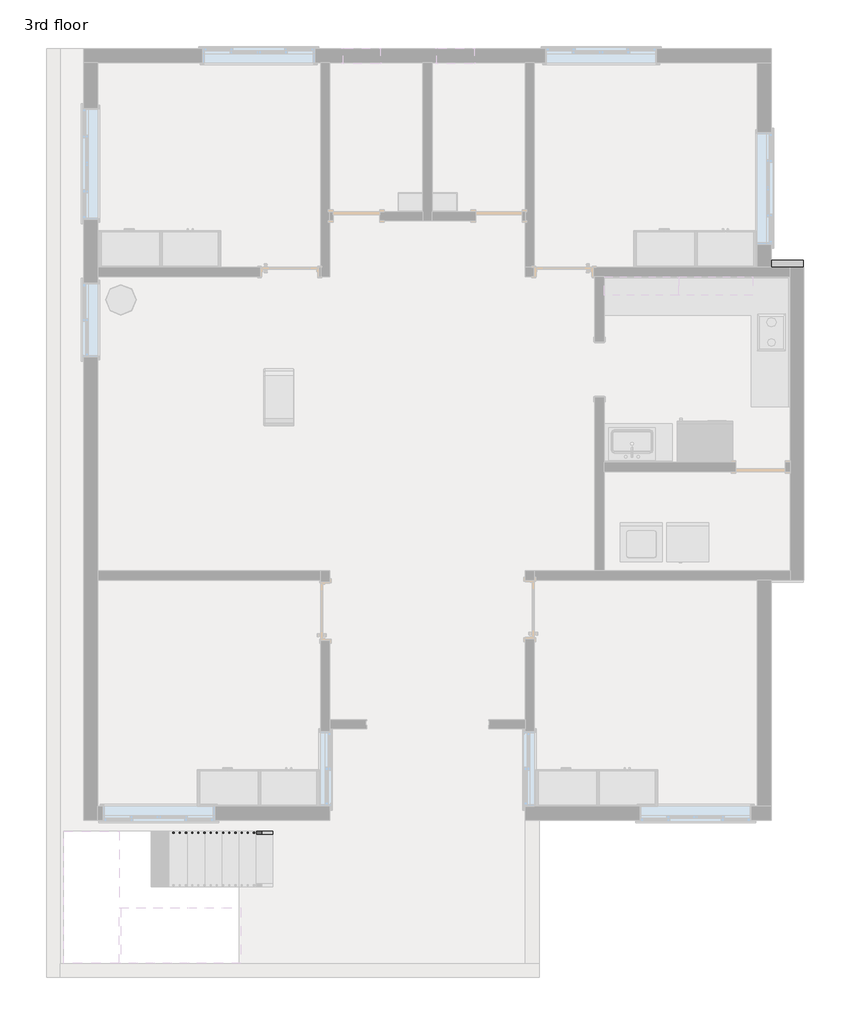
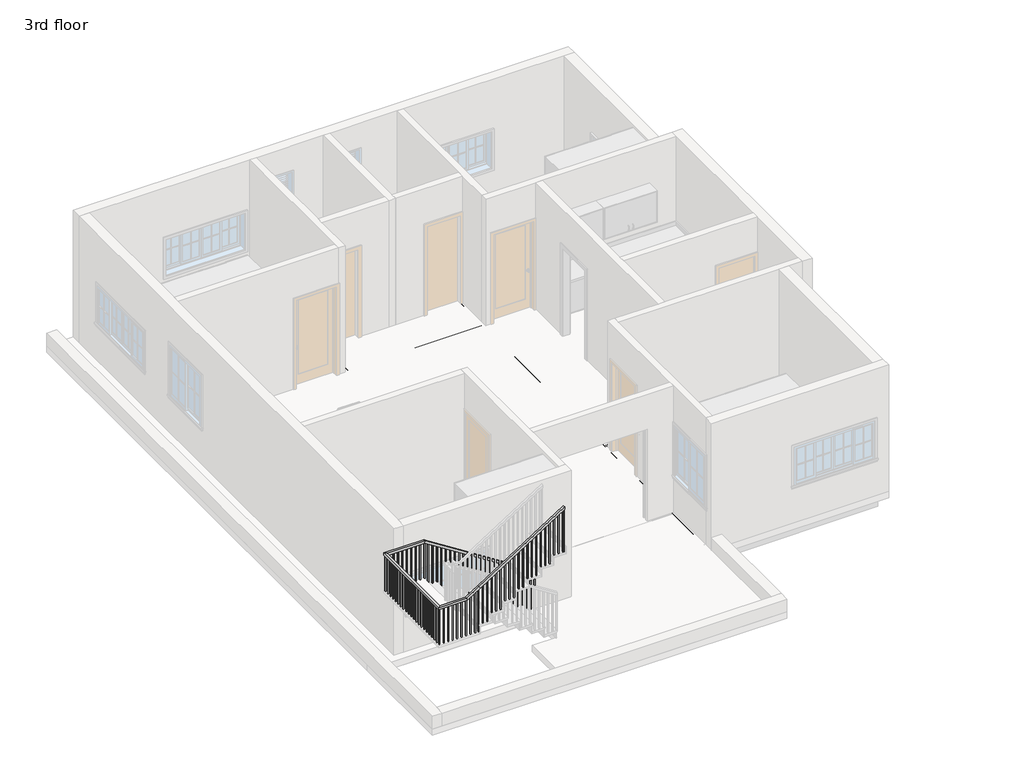
# One storey, part 2 of 4: 6 beams, 1 railing.
"""IFC4 building model written with IfcOpenShell, lengths in millimetres."""

from ifc_helpers import new_model, si_unit, frame, origin, place, context, project, spatial, polyline, outline, extrude, faceted_brep, element, save

model = new_model("IFC4")

# Units and contexts
model_context = context("Model", 3, world=origin())
ifc_project = project(units=[si_unit("LENGTHUNIT", "METRE", prefix="MILLI")], contexts=[model_context])

# Site, building, storey
site = spatial("IfcSite", under=ifc_project)
building = spatial("IfcBuilding", under=site)
storey = spatial("IfcBuildingStorey", under=building, Name="3rd floor", Elevation=10210.8)

# Beams
placement = place(None, origin())
element("IfcBeam", 1, ObjectType="Concrete-Rectangular Beam", at=placement, inside=storey, context=model_context, shape_type="Brep", body=[
    faceted_brep([(-12413.6124084, 10142.6961804, 10210.8), (-12413.6124084, 9914.0961804, 10210.8), (-8794.1124084, 9914.0961804, 10210.8), (-8565.5124084, 9914.0961804, 10210.8), (-7117.7124084, 9914.0961804, 10210.8), (-6889.1124084, 9914.0961804, 10210.8), (-5441.3124084, 9914.0961804, 10210.8), (-5212.7124084, 9914.0961804, 10210.8), (-1593.2124084, 9914.0961804, 10210.8), (-1593.2124084, 10142.6961804, 10210.8), (-5174.6124084, 10142.6961804, 10210.8), (-5174.6124084, 9952.1961804, 10210.8), (-5479.4124084, 9952.1961804, 10210.8), (-5479.4124084, 10142.6961804, 10210.8), (-8451.2124084, 10142.6961804, 10210.8), (-8451.2124084, 9952.1961804, 10210.8), (-8756.0124084, 9952.1961804, 10210.8), (-8756.0124084, 10142.6961804, 10210.8), (-12413.6124084, 9914.0961804, 9906.0), (-8794.1124084, 9914.0961804, 9906.0), (-8565.5124084, 9914.0961804, 9906.0), (-7117.7124084, 9914.0961804, 9906.0), (-6889.1124084, 9914.0961804, 9906.0), (-5441.3124084, 9914.0961804, 9906.0), (-5212.7124084, 9914.0961804, 9906.0), (-1593.2124084, 9914.0961804, 9906.0), (-12413.6124084, 10142.6961804, 9906.0), (-8756.0124084, 10142.6961804, 9906.0), (-8756.0124084, 9952.1961804, 9906.0), (-8451.2124084, 9952.1961804, 9906.0), (-8451.2124084, 10142.6961804, 9906.0), (-5479.4124084, 10142.6961804, 9906.0), (-5479.4124084, 9952.1961804, 9906.0), (-5174.6124084, 9952.1961804, 9906.0), (-5174.6124084, 10142.6961804, 9906.0), (-1593.2124084, 10142.6961804, 9906.0)], [[[0, 1, 2, 3, 4, 5, 6, 7, 8, 9, 10, 11, 12, 13, 14, 15, 16, 17]], [[1, 18, 19, 20, 21, 22, 23, 24, 25, 8, 7, 6, 5, 4, 3, 2]], [[18, 26, 27, 28, 29, 30, 31, 32, 33, 34, 35, 25, 24, 23, 22, 21, 20, 19]], [[26, 0, 17, 27]], [[1, 0, 26, 18]], [[9, 8, 25, 35]], [[15, 14, 30, 29]], [[16, 15, 29, 28]], [[17, 16, 28, 27]], [[9, 35, 34, 10]], [[33, 11, 10, 34]], [[11, 33, 32, 12]], [[12, 32, 31, 13]], [[30, 14, 13, 31]]]),
])
element("IfcBeam", 2, ObjectType="Concrete-Rectangular Beam", at=placement, inside=storey, context=model_context, shape_type="SweptSolid", body=[
    extrude(outline(polyline([(-1593.2124084, 9875.9961804), (-1364.6124084, 9875.9961804), (-1364.6124084, 6751.7961804), (-1593.2124084, 6751.7961804), (-1593.2124084, 9875.9961804)])), frame((0.0, 0.0, 9906.0), z_axis=(0.0, 0.0, 1.0), x_axis=(1.0, 0.0, 0.0)), (0.0, 0.0, 1.0), 304.8),
])
element("IfcBeam", 3, ObjectType="Concrete-Rectangular Beam", at=placement, inside=storey, context=model_context, shape_type="Brep", body=[
    faceted_brep([(-843.9124084, 6713.6961804, 10210.8), (-843.9124084, 6485.0961804, 10210.8), (-843.9124084, 6485.0961804, 9906.0), (-843.9124084, 6713.6961804, 9906.0), (-1364.6124084, 6713.6961804, 10210.8), (-1364.6124084, 6485.0961804, 10210.8), (-1364.6124084, 6485.0961804, 9906.0), (-1364.6124084, 6713.6961804, 9906.0)], [[[0, 1, 2, 3]], [[1, 0, 4, 5]], [[2, 1, 5, 6]], [[3, 2, 6, 7]], [[0, 3, 7, 4]], [[5, 4, 7, 6]]]),
    faceted_brep([(-12413.6124084, 6485.0961804, 10210.8), (-12413.6124084, 6713.6961804, 10210.8), (-12413.6124084, 6713.6961804, 9906.0), (-12413.6124084, 6485.0961804, 9906.0), (-8756.0124084, 6713.6961804, 10210.8), (-8756.0124084, 6485.0961804, 10210.8), (-8756.0124084, 6485.0961804, 9906.0), (-8756.0124084, 6713.6961804, 9906.0), (-8794.1124084, 6485.0961804, 10210.8), (-8794.1124084, 6713.6961804, 10210.8), (-8794.1124084, 6485.0961804, 9906.0), (-8794.1124084, 6713.6961804, 9906.0)], [[[0, 1, 2, 3]], [[4, 5, 6, 7]], [[1, 0, 8, 5, 4, 9]], [[0, 3, 10, 6, 5, 8]], [[3, 2, 11, 7, 6, 10]], [[2, 1, 9, 4, 7, 11]]]),
    faceted_brep([(-1593.2124084, 6713.6961804, 10210.8), (-1593.2124084, 6485.0961804, 10210.8), (-1593.2124084, 6485.0961804, 9906.0), (-1593.2124084, 6713.6961804, 9906.0), (-5212.7124084, 6713.6961804, 10210.8), (-5250.8124084, 6713.6961804, 10210.8), (-5250.8124084, 6485.0961804, 10210.8), (-5212.7124084, 6485.0961804, 10210.8), (-5250.8124084, 6485.0961804, 9906.0), (-5212.7124084, 6485.0961804, 9906.0), (-5250.8124084, 6713.6961804, 9906.0), (-5212.7124084, 6713.6961804, 9906.0)], [[[0, 1, 2, 3]], [[1, 0, 4, 5, 6, 7]], [[2, 1, 7, 6, 8, 9]], [[3, 2, 9, 8, 10, 11]], [[0, 3, 11, 10, 5, 4]], [[6, 5, 10, 8]]]),
    faceted_brep([(-8527.4124084, 6485.0961804, 10210.8), (-8527.4124084, 6713.6961804, 10210.8), (-8527.4124084, 6713.6961804, 9906.0), (-8527.4124084, 6485.0961804, 9906.0), (-5479.4124084, 6713.6961804, 10210.8), (-5479.4124084, 6485.0961804, 10210.8), (-5479.4124084, 6485.0961804, 9906.0), (-5479.4124084, 6713.6961804, 9906.0)], [[[0, 1, 2, 3]], [[4, 5, 6, 7]], [[1, 0, 5, 4]], [[0, 3, 6, 5]], [[3, 2, 7, 6]], [[2, 1, 4, 7]]]),
])
element("IfcBeam", 4, ObjectType="Concrete-Rectangular Beam", at=placement, inside=storey, context=model_context, shape_type="Brep", body=[
    faceted_brep([(-5212.7124084, 9914.0961804, 10210.8), (-5441.3124084, 9914.0961804, 10210.8), (-5441.3124084, 7551.8961804, 10210.8), (-5441.3124084, 7323.2961804, 10210.8), (-5441.3124084, 6751.7961804, 10210.8), (-5250.8124084, 6751.7961804, 10210.8), (-5250.8124084, 6713.6961804, 10210.8), (-5212.7124084, 6713.6961804, 10210.8), (-5212.7124084, 9914.0961804, 9906.0), (-5212.7124084, 6713.6961804, 9906.0), (-5441.3124084, 9914.0961804, 9906.0), (-5250.8124084, 6713.6961804, 9906.0), (-5250.8124084, 6751.7961804, 9906.0), (-5441.3124084, 6751.7961804, 9906.0), (-5441.3124084, 7323.2961804, 9906.0), (-5441.3124084, 7551.8961804, 9906.0)], [[[0, 1, 2, 3, 4, 5, 6, 7]], [[8, 0, 7, 9]], [[10, 8, 9, 11, 12, 13, 14, 15]], [[1, 10, 15, 14, 13, 4, 3, 2]], [[1, 0, 8, 10]], [[9, 7, 6, 11]], [[5, 4, 13, 12]], [[6, 5, 12, 11]]]),
    faceted_brep([(-5212.7124084, -2201.7038196, 10210.8), (-5441.3124084, -2201.7038196, 10210.8), (-5441.3124084, -2201.7038196, 9906.0), (-5212.7124084, -2201.7038196, 9906.0), (-5441.3124084, 1430.4961804, 9906.0), (-5441.3124084, 1430.4961804, 10210.8), (-5212.7124084, 1430.4961804, 10210.8), (-5212.7124084, 1430.4961804, 9906.0), (-5441.3124084, -779.3038196, 9906.0), (-5441.3124084, -1007.9038196, 9906.0), (-5441.3124084, -1007.9038196, 10210.8), (-5441.3124084, -779.3038196, 10210.8)], [[[0, 1, 2, 3]], [[4, 5, 6, 7]], [[5, 4, 8, 9, 2, 1, 10, 11]], [[1, 0, 6, 5, 11, 10]], [[0, 3, 7, 6]], [[3, 2, 9, 8, 4, 7]]]),
    faceted_brep([(-5212.7124084, 6485.0961804, 10210.8), (-5212.7124084, 6485.0961804, 9906.0), (-5250.8124084, 6485.0961804, 9906.0), (-5250.8124084, 6485.0961804, 10210.8), (-5250.8124084, 6446.9961804, 10210.8), (-5441.3124084, 6446.9961804, 10210.8), (-5441.3124084, 1659.0961804, 10210.8), (-5403.2124084, 1659.0961804, 10210.8), (-5403.2124084, 1697.1961804, 10210.8), (-5212.7124084, 1697.1961804, 10210.8), (-5212.7124084, 1697.1961804, 9906.0), (-5403.2124084, 1697.1961804, 9906.0), (-5403.2124084, 1659.0961804, 9906.0), (-5441.3124084, 1659.0961804, 9906.0), (-5441.3124084, 6446.9961804, 9906.0), (-5250.8124084, 6446.9961804, 9906.0)], [[[0, 1, 2, 3]], [[0, 3, 4, 5, 6, 7, 8, 9]], [[1, 0, 9, 10]], [[2, 1, 10, 11, 12, 13, 14, 15]], [[6, 13, 12, 7]], [[13, 6, 5, 14]], [[3, 2, 15, 4]], [[5, 4, 15, 14]], [[8, 11, 10, 9]], [[11, 8, 7, 12]]]),
])
element("IfcBeam", 5, ObjectType="Concrete-Rectangular Beam", at=placement, inside=storey, context=model_context, shape_type="SweptSolid", body=[
    extrude(outline(polyline([(-7117.7124084, 9914.0961804), (-6889.1124084, 9914.0961804), (-6889.1124084, 7551.8961804), (-7117.7124084, 7551.8961804), (-7117.7124084, 9914.0961804)])), frame((0.0, 0.0, 9906.0), z_axis=(0.0, 0.0, 1.0), x_axis=(1.0, 0.0, 0.0)), (0.0, 0.0, 1.0), 304.8),
])
element("IfcBeam", 6, ObjectType="Concrete-Rectangular Beam", at=placement, inside=storey, context=model_context, shape_type="Brep", body=[
    faceted_brep([(-5441.3124084, 7323.2961804, 10210.8), (-5441.3124084, 7551.8961804, 10210.8), (-6889.1124084, 7551.8961804, 10210.8), (-7117.7124084, 7551.8961804, 10210.8), (-8565.5124084, 7551.8961804, 10210.8), (-8565.5124084, 7323.2961804, 10210.8), (-5441.3124084, 7323.2961804, 9906.0), (-8565.5124084, 7323.2961804, 9906.0), (-5441.3124084, 7551.8961804, 9906.0), (-8565.5124084, 7551.8961804, 9906.0), (-7117.7124084, 7551.8961804, 9906.0), (-6889.1124084, 7551.8961804, 9906.0)], [[[0, 1, 2, 3, 4, 5]], [[6, 0, 5, 7]], [[8, 6, 7, 9, 10, 11]], [[1, 8, 11, 10, 9, 4, 3, 2]], [[1, 0, 6, 8]], [[5, 4, 9, 7]]]),
])

# Railing
element("IfcRailing", 7, ObjectType="Handrail - Rectangular", at=placement, inside=storey, context=model_context, shape_type="SolidModel", body=[
    faceted_brep([(-9543.8120641, -2698.7669819, 11303.0), (-9543.8120641, -2698.7669819, 11242.786276), (-9543.8120641, -2647.9669819, 11242.786276), (-9543.8120641, -2647.9669819, 11303.0), (-12058.4120641, -2698.7669819, 12903.2), (-12073.205059, -2698.7669819, 12852.4), (-12073.205059, -2647.9669819, 12852.4), (-12058.4120641, -2647.9669819, 12903.2), (-12922.0120641, -2698.7669819, 12903.2), (-12922.0120641, -2698.7669819, 12852.4), (-12972.8120641, -2647.9669819, 12852.4), (-12972.8120641, -2647.9669819, 12903.2), (-12922.0120641, -4767.1038196, 12903.2), (-12922.0120641, -4767.1038196, 12852.4), (-12972.8120641, -4817.9038196, 12852.4), (-12972.8120641, -4817.9038196, 12903.2), (-12337.8120641, -4767.1038196, 12903.2), (-12323.0190691, -4767.1038196, 12852.4), (-12323.0190691, -4817.9038196, 12852.4), (-12337.8120641, -4817.9038196, 12903.2), (-12058.4120641, -4767.1038196, 13081.0), (-12031.138789, -4767.1038196, 13038.1419964), (-12031.138789, -4817.9038196, 13038.1419964), (-12058.4120641, -4817.9038196, 13081.0), (-10102.6120641, -4767.1038196, 14325.6), (-10102.6120641, -4817.9038196, 14325.6), (-10102.6120641, -4817.9038196, 14265.386276), (-10102.6120641, -4767.1038196, 14265.386276)], [[[0, 1, 2, 3]], [[1, 0, 4, 5]], [[2, 1, 5, 6]], [[3, 2, 6, 7]], [[0, 3, 7, 4]], [[5, 4, 8, 9]], [[6, 5, 9, 10]], [[7, 6, 10, 11]], [[4, 7, 11, 8]], [[9, 8, 12, 13]], [[10, 9, 13, 14]], [[11, 10, 14, 15]], [[8, 11, 15, 12]], [[13, 12, 16, 17]], [[14, 13, 17, 18]], [[15, 14, 18, 19]], [[12, 15, 19, 16]], [[17, 16, 20, 21]], [[18, 17, 21, 22]], [[19, 18, 22, 23]], [[16, 19, 23, 20]], [[24, 25, 26, 27]], [[21, 20, 24, 27]], [[22, 21, 27, 26]], [[23, 22, 26, 25]], [[20, 23, 25, 24]]]),
    extrude(outline(polyline([(14255.2840032, -10118.4870641), (14243.161276, -10137.5370641), (13233.4, -10137.5370641), (13233.4, -10118.4870641), (14255.2840032, -10118.4870641)])), frame((0.0, -4802.0288196, 0.0), z_axis=(0.0, 1.0, 0.0), x_axis=(0.0, 0.0, 1.0)), (0.0, 0.0, 1.0), 19.05),
    extrude(outline(polyline([(14190.6294578, -10220.0870641), (14178.5067305, -10239.1370641), (13233.4, -10239.1370641), (13233.4, -10220.0870641), (14190.6294578, -10220.0870641)])), frame((0.0, -4802.0288196, 0.0), z_axis=(0.0, 1.0, 0.0), x_axis=(0.0, 0.0, 1.0)), (0.0, 0.0, 1.0), 19.05),
    extrude(outline(polyline([(14125.9749123, -10321.6870641), (14113.8521851, -10340.7370641), (13233.4, -10340.7370641), (13233.4, -10321.6870641), (14125.9749123, -10321.6870641)])), frame((0.0, -4802.0288196, 0.0), z_axis=(0.0, 1.0, 0.0), x_axis=(0.0, 0.0, 1.0)), (0.0, 0.0, 1.0), 19.05),
    extrude(outline(polyline([(14061.3203669, -10423.2870641), (14049.1976396, -10442.3370641), (13055.6, -10442.3370641), (13055.6, -10423.2870641), (14061.3203669, -10423.2870641)])), frame((0.0, -4802.0288196, 0.0), z_axis=(0.0, 1.0, 0.0), x_axis=(0.0, 0.0, 1.0)), (0.0, 0.0, 1.0), 19.05),
    extrude(outline(polyline([(13996.6658214, -10524.8870641), (13984.5430941, -10543.9370641), (13055.6, -10543.9370641), (13055.6, -10524.8870641), (13996.6658214, -10524.8870641)])), frame((0.0, -4802.0288196, 0.0), z_axis=(0.0, 1.0, 0.0), x_axis=(0.0, 0.0, 1.0)), (0.0, 0.0, 1.0), 19.05),
    extrude(outline(polyline([(13932.011276, -10626.4870641), (13919.8885487, -10645.5370641), (13055.6, -10645.5370641), (13055.6, -10626.4870641), (13932.011276, -10626.4870641)])), frame((0.0, -4802.0288196, 0.0), z_axis=(0.0, 1.0, 0.0), x_axis=(0.0, 0.0, 1.0)), (0.0, 0.0, 1.0), 19.05),
    extrude(outline(polyline([(13867.3567305, -10728.0870641), (13855.2340032, -10747.1370641), (12877.8, -10747.1370641), (12877.8, -10728.0870641), (13867.3567305, -10728.0870641)])), frame((0.0, -4802.0288196, 0.0), z_axis=(0.0, 1.0, 0.0), x_axis=(0.0, 0.0, 1.0)), (0.0, 0.0, 1.0), 19.05),
    extrude(outline(polyline([(13802.7021851, -10829.6870641), (13790.5794578, -10848.7370641), (12877.8, -10848.7370641), (12877.8, -10829.6870641), (13802.7021851, -10829.6870641)])), frame((0.0, -4802.0288196, 0.0), z_axis=(0.0, 1.0, 0.0), x_axis=(0.0, 0.0, 1.0)), (0.0, 0.0, 1.0), 19.05),
    extrude(outline(polyline([(13738.0476396, -10931.2870641), (13725.9249123, -10950.3370641), (12877.8, -10950.3370641), (12877.8, -10931.2870641), (13738.0476396, -10931.2870641)])), frame((0.0, -4802.0288196, 0.0), z_axis=(0.0, 1.0, 0.0), x_axis=(0.0, 0.0, 1.0)), (0.0, 0.0, 1.0), 19.05),
    extrude(outline(polyline([(13673.3930941, -11032.8870641), (13661.2703669, -11051.9370641), (12700.0, -11051.9370641), (12700.0, -11032.8870641), (13673.3930941, -11032.8870641)])), frame((0.0, -4802.0288196, 0.0), z_axis=(0.0, 1.0, 0.0), x_axis=(0.0, 0.0, 1.0)), (0.0, 0.0, 1.0), 19.05),
    extrude(outline(polyline([(13608.7385487, -11134.4870641), (13596.6158214, -11153.5370641), (12700.0, -11153.5370641), (12700.0, -11134.4870641), (13608.7385487, -11134.4870641)])), frame((0.0, -4802.0288196, 0.0), z_axis=(0.0, 1.0, 0.0), x_axis=(0.0, 0.0, 1.0)), (0.0, 0.0, 1.0), 19.05),
    extrude(outline(polyline([(13544.0840032, -11236.0870641), (13531.961276, -11255.1370641), (12522.2, -11255.1370641), (12522.2, -11236.0870641), (13544.0840032, -11236.0870641)])), frame((0.0, -4802.0288196, 0.0), z_axis=(0.0, 1.0, 0.0), x_axis=(0.0, 0.0, 1.0)), (0.0, 0.0, 1.0), 19.05),
    extrude(outline(polyline([(13479.4294578, -11337.6870641), (13467.3067305, -11356.7370641), (12522.2, -11356.7370641), (12522.2, -11337.6870641), (13479.4294578, -11337.6870641)])), frame((0.0, -4802.0288196, 0.0), z_axis=(0.0, 1.0, 0.0), x_axis=(0.0, 0.0, 1.0)), (0.0, 0.0, 1.0), 19.05),
    extrude(outline(polyline([(13414.7749123, -11439.2870641), (13402.6521851, -11458.3370641), (12522.2, -11458.3370641), (12522.2, -11439.2870641), (13414.7749123, -11439.2870641)])), frame((0.0, -4802.0288196, 0.0), z_axis=(0.0, 1.0, 0.0), x_axis=(0.0, 0.0, 1.0)), (0.0, 0.0, 1.0), 19.05),
    extrude(outline(polyline([(13350.1203669, -11540.8870641), (13337.9976396, -11559.9370641), (12344.4, -11559.9370641), (12344.4, -11540.8870641), (13350.1203669, -11540.8870641)])), frame((0.0, -4802.0288196, 0.0), z_axis=(0.0, 1.0, 0.0), x_axis=(0.0, 0.0, 1.0)), (0.0, 0.0, 1.0), 19.05),
    extrude(outline(polyline([(13285.4658214, -11642.4870641), (13273.3430941, -11661.5370641), (12344.4, -11661.5370641), (12344.4, -11642.4870641), (13285.4658214, -11642.4870641)])), frame((0.0, -4802.0288196, 0.0), z_axis=(0.0, 1.0, 0.0), x_axis=(0.0, 0.0, 1.0)), (0.0, 0.0, 1.0), 19.05),
    extrude(outline(polyline([(13220.811276, -11744.0870641), (13208.6885487, -11763.1370641), (12344.4, -11763.1370641), (12344.4, -11744.0870641), (13220.811276, -11744.0870641)])), frame((0.0, -4802.0288196, 0.0), z_axis=(0.0, 1.0, 0.0), x_axis=(0.0, 0.0, 1.0)), (0.0, 0.0, 1.0), 19.05),
    extrude(outline(polyline([(13156.1567305, -11845.6870641), (13144.0340032, -11864.7370641), (12166.6, -11864.7370641), (12166.6, -11845.6870641), (13156.1567305, -11845.6870641)])), frame((0.0, -4802.0288196, 0.0), z_axis=(0.0, 1.0, 0.0), x_axis=(0.0, 0.0, 1.0)), (0.0, 0.0, 1.0), 19.05),
    extrude(outline(polyline([(13091.5021851, -11947.2870641), (13079.3794578, -11966.3370641), (12166.6, -11966.3370641), (12166.6, -11947.2870641), (13091.5021851, -11947.2870641)])), frame((0.0, -4802.0288196, 0.0), z_axis=(0.0, 1.0, 0.0), x_axis=(0.0, 0.0, 1.0)), (0.0, 0.0, 1.0), 19.05),
    extrude(outline(polyline([(12978.3567305, -12125.0870641), (12966.2340032, -12144.1370641), (11988.8, -12144.1370641), (11988.8, -12125.0870641), (12978.3567305, -12125.0870641)])), frame((0.0, -4802.0288196, 0.0), z_axis=(0.0, 1.0, 0.0), x_axis=(0.0, 0.0, 1.0)), (0.0, 0.0, 1.0), 19.05),
    extrude(outline(polyline([(12913.7021851, -12226.6870641), (12901.5794578, -12245.7370641), (11988.8, -12245.7370641), (11988.8, -12226.6870641), (12913.7021851, -12226.6870641)])), frame((0.0, -4802.0288196, 0.0), z_axis=(0.0, 1.0, 0.0), x_axis=(0.0, 0.0, 1.0)), (0.0, 0.0, 1.0), 19.05),
    extrude(outline(polyline([(-12347.3370641, -4802.0288196), (-12347.3370641, -4782.9788196), (-12328.2870641, -4782.9788196), (-12328.2870641, -4802.0288196), (-12347.3370641, -4802.0288196)])), frame((0.0, 0.0, 11988.8), z_axis=(0.0, 0.0, 1.0), x_axis=(1.0, 0.0, 0.0)), (0.0, 0.0, 1.0), 863.6),
    extrude(outline(polyline([(-12448.9370641, -4802.0288196), (-12448.9370641, -4782.9788196), (-12429.8870641, -4782.9788196), (-12429.8870641, -4802.0288196), (-12448.9370641, -4802.0288196)])), frame((0.0, 0.0, 11988.8), z_axis=(0.0, 0.0, 1.0), x_axis=(1.0, 0.0, 0.0)), (0.0, 0.0, 1.0), 863.6),
    extrude(outline(polyline([(-12550.5370641, -4802.0288196), (-12550.5370641, -4782.9788196), (-12531.4870641, -4782.9788196), (-12531.4870641, -4802.0288196), (-12550.5370641, -4802.0288196)])), frame((0.0, 0.0, 11988.8), z_axis=(0.0, 0.0, 1.0), x_axis=(1.0, 0.0, 0.0)), (0.0, 0.0, 1.0), 863.6),
    extrude(outline(polyline([(-12652.1370641, -4802.0288196), (-12652.1370641, -4782.9788196), (-12633.0870641, -4782.9788196), (-12633.0870641, -4802.0288196), (-12652.1370641, -4802.0288196)])), frame((0.0, 0.0, 11988.8), z_axis=(0.0, 0.0, 1.0), x_axis=(1.0, 0.0, 0.0)), (0.0, 0.0, 1.0), 863.6),
    extrude(outline(polyline([(-12753.7370641, -4802.0288196), (-12753.7370641, -4782.9788196), (-12734.6870641, -4782.9788196), (-12734.6870641, -4802.0288196), (-12753.7370641, -4802.0288196)])), frame((0.0, 0.0, 11988.8), z_axis=(0.0, 0.0, 1.0), x_axis=(1.0, 0.0, 0.0)), (0.0, 0.0, 1.0), 863.6),
    extrude(outline(polyline([(-12855.3370641, -4802.0288196), (-12855.3370641, -4782.9788196), (-12836.2870641, -4782.9788196), (-12836.2870641, -4802.0288196), (-12855.3370641, -4802.0288196)])), frame((0.0, 0.0, 11988.8), z_axis=(0.0, 0.0, 1.0), x_axis=(1.0, 0.0, 0.0)), (0.0, 0.0, 1.0), 863.6),
    extrude(outline(polyline([(-12956.9370641, -4695.8419819), (-12937.8870641, -4695.8419819), (-12937.8870641, -4714.8919819), (-12956.9370641, -4714.8919819), (-12956.9370641, -4695.8419819)])), frame((0.0, 0.0, 11988.8), z_axis=(0.0, 0.0, 1.0), x_axis=(1.0, 0.0, 0.0)), (0.0, 0.0, 1.0), 863.6),
    extrude(outline(polyline([(-12956.9370641, -4594.2419819), (-12937.8870641, -4594.2419819), (-12937.8870641, -4613.2919819), (-12956.9370641, -4613.2919819), (-12956.9370641, -4594.2419819)])), frame((0.0, 0.0, 11988.8), z_axis=(0.0, 0.0, 1.0), x_axis=(1.0, 0.0, 0.0)), (0.0, 0.0, 1.0), 863.6),
    extrude(outline(polyline([(-12956.9370641, -4492.6419819), (-12937.8870641, -4492.6419819), (-12937.8870641, -4511.6919819), (-12956.9370641, -4511.6919819), (-12956.9370641, -4492.6419819)])), frame((0.0, 0.0, 11988.8), z_axis=(0.0, 0.0, 1.0), x_axis=(1.0, 0.0, 0.0)), (0.0, 0.0, 1.0), 863.6),
    extrude(outline(polyline([(-12956.9370641, -4391.0419819), (-12937.8870641, -4391.0419819), (-12937.8870641, -4410.0919819), (-12956.9370641, -4410.0919819), (-12956.9370641, -4391.0419819)])), frame((0.0, 0.0, 11988.8), z_axis=(0.0, 0.0, 1.0), x_axis=(1.0, 0.0, 0.0)), (0.0, 0.0, 1.0), 863.6),
    extrude(outline(polyline([(-12956.9370641, -4289.4419819), (-12937.8870641, -4289.4419819), (-12937.8870641, -4308.4919819), (-12956.9370641, -4308.4919819), (-12956.9370641, -4289.4419819)])), frame((0.0, 0.0, 11988.8), z_axis=(0.0, 0.0, 1.0), x_axis=(1.0, 0.0, 0.0)), (0.0, 0.0, 1.0), 863.6),
    extrude(outline(polyline([(-12956.9370641, -4187.8419819), (-12937.8870641, -4187.8419819), (-12937.8870641, -4206.8919819), (-12956.9370641, -4206.8919819), (-12956.9370641, -4187.8419819)])), frame((0.0, 0.0, 11988.8), z_axis=(0.0, 0.0, 1.0), x_axis=(1.0, 0.0, 0.0)), (0.0, 0.0, 1.0), 863.6),
    extrude(outline(polyline([(-12956.9370641, -4086.2419819), (-12937.8870641, -4086.2419819), (-12937.8870641, -4105.2919819), (-12956.9370641, -4105.2919819), (-12956.9370641, -4086.2419819)])), frame((0.0, 0.0, 11988.8), z_axis=(0.0, 0.0, 1.0), x_axis=(1.0, 0.0, 0.0)), (0.0, 0.0, 1.0), 863.6),
    extrude(outline(polyline([(-12956.9370641, -3984.6419819), (-12937.8870641, -3984.6419819), (-12937.8870641, -4003.6919819), (-12956.9370641, -4003.6919819), (-12956.9370641, -3984.6419819)])), frame((0.0, 0.0, 11988.8), z_axis=(0.0, 0.0, 1.0), x_axis=(1.0, 0.0, 0.0)), (0.0, 0.0, 1.0), 863.6),
    extrude(outline(polyline([(-12956.9370641, -3883.0419819), (-12937.8870641, -3883.0419819), (-12937.8870641, -3902.0919819), (-12956.9370641, -3902.0919819), (-12956.9370641, -3883.0419819)])), frame((0.0, 0.0, 11988.8), z_axis=(0.0, 0.0, 1.0), x_axis=(1.0, 0.0, 0.0)), (0.0, 0.0, 1.0), 863.6),
    extrude(outline(polyline([(-12956.9370641, -3781.4419819), (-12937.8870641, -3781.4419819), (-12937.8870641, -3800.4919819), (-12956.9370641, -3800.4919819), (-12956.9370641, -3781.4419819)])), frame((0.0, 0.0, 11988.8), z_axis=(0.0, 0.0, 1.0), x_axis=(1.0, 0.0, 0.0)), (0.0, 0.0, 1.0), 863.6),
    extrude(outline(polyline([(-12956.9370641, -3679.8419819), (-12937.8870641, -3679.8419819), (-12937.8870641, -3698.8919819), (-12956.9370641, -3698.8919819), (-12956.9370641, -3679.8419819)])), frame((0.0, 0.0, 11988.8), z_axis=(0.0, 0.0, 1.0), x_axis=(1.0, 0.0, 0.0)), (0.0, 0.0, 1.0), 863.6),
    extrude(outline(polyline([(-12956.9370641, -3578.2419819), (-12937.8870641, -3578.2419819), (-12937.8870641, -3597.2919819), (-12956.9370641, -3597.2919819), (-12956.9370641, -3578.2419819)])), frame((0.0, 0.0, 11988.8), z_axis=(0.0, 0.0, 1.0), x_axis=(1.0, 0.0, 0.0)), (0.0, 0.0, 1.0), 863.6),
    extrude(outline(polyline([(-12956.9370641, -3476.6419819), (-12937.8870641, -3476.6419819), (-12937.8870641, -3495.6919819), (-12956.9370641, -3495.6919819), (-12956.9370641, -3476.6419819)])), frame((0.0, 0.0, 11988.8), z_axis=(0.0, 0.0, 1.0), x_axis=(1.0, 0.0, 0.0)), (0.0, 0.0, 1.0), 863.6),
    extrude(outline(polyline([(-12956.9370641, -3375.0419819), (-12937.8870641, -3375.0419819), (-12937.8870641, -3394.0919819), (-12956.9370641, -3394.0919819), (-12956.9370641, -3375.0419819)])), frame((0.0, 0.0, 11988.8), z_axis=(0.0, 0.0, 1.0), x_axis=(1.0, 0.0, 0.0)), (0.0, 0.0, 1.0), 863.6),
    extrude(outline(polyline([(-12956.9370641, -3273.4419819), (-12937.8870641, -3273.4419819), (-12937.8870641, -3292.4919819), (-12956.9370641, -3292.4919819), (-12956.9370641, -3273.4419819)])), frame((0.0, 0.0, 11988.8), z_axis=(0.0, 0.0, 1.0), x_axis=(1.0, 0.0, 0.0)), (0.0, 0.0, 1.0), 863.6),
    extrude(outline(polyline([(-12956.9370641, -3171.8419819), (-12937.8870641, -3171.8419819), (-12937.8870641, -3190.8919819), (-12956.9370641, -3190.8919819), (-12956.9370641, -3171.8419819)])), frame((0.0, 0.0, 11988.8), z_axis=(0.0, 0.0, 1.0), x_axis=(1.0, 0.0, 0.0)), (0.0, 0.0, 1.0), 863.6),
    extrude(outline(polyline([(-12956.9370641, -3070.2419819), (-12937.8870641, -3070.2419819), (-12937.8870641, -3089.2919819), (-12956.9370641, -3089.2919819), (-12956.9370641, -3070.2419819)])), frame((0.0, 0.0, 11988.8), z_axis=(0.0, 0.0, 1.0), x_axis=(1.0, 0.0, 0.0)), (0.0, 0.0, 1.0), 863.6),
    extrude(outline(polyline([(-12956.9370641, -2968.6419819), (-12937.8870641, -2968.6419819), (-12937.8870641, -2987.6919819), (-12956.9370641, -2987.6919819), (-12956.9370641, -2968.6419819)])), frame((0.0, 0.0, 11988.8), z_axis=(0.0, 0.0, 1.0), x_axis=(1.0, 0.0, 0.0)), (0.0, 0.0, 1.0), 863.6),
    extrude(outline(polyline([(-12956.9370641, -2867.0419819), (-12937.8870641, -2867.0419819), (-12937.8870641, -2886.0919819), (-12956.9370641, -2886.0919819), (-12956.9370641, -2867.0419819)])), frame((0.0, 0.0, 11988.8), z_axis=(0.0, 0.0, 1.0), x_axis=(1.0, 0.0, 0.0)), (0.0, 0.0, 1.0), 863.6),
    extrude(outline(polyline([(-12956.9370641, -2765.4419819), (-12937.8870641, -2765.4419819), (-12937.8870641, -2784.4919819), (-12956.9370641, -2784.4919819), (-12956.9370641, -2765.4419819)])), frame((0.0, 0.0, 11988.8), z_axis=(0.0, 0.0, 1.0), x_axis=(1.0, 0.0, 0.0)), (0.0, 0.0, 1.0), 863.6),
    extrude(outline(polyline([(-12861.6870641, -2663.8419819), (-12861.6870641, -2682.8919819), (-12880.7370641, -2682.8919819), (-12880.7370641, -2663.8419819), (-12861.6870641, -2663.8419819)])), frame((0.0, 0.0, 11988.8), z_axis=(0.0, 0.0, 1.0), x_axis=(1.0, 0.0, 0.0)), (0.0, 0.0, 1.0), 863.6),
    extrude(outline(polyline([(-12760.0870641, -2663.8419819), (-12760.0870641, -2682.8919819), (-12779.1370641, -2682.8919819), (-12779.1370641, -2663.8419819), (-12760.0870641, -2663.8419819)])), frame((0.0, 0.0, 11988.8), z_axis=(0.0, 0.0, 1.0), x_axis=(1.0, 0.0, 0.0)), (0.0, 0.0, 1.0), 863.6),
    extrude(outline(polyline([(-12658.4870641, -2663.8419819), (-12658.4870641, -2682.8919819), (-12677.5370641, -2682.8919819), (-12677.5370641, -2663.8419819), (-12658.4870641, -2663.8419819)])), frame((0.0, 0.0, 11988.8), z_axis=(0.0, 0.0, 1.0), x_axis=(1.0, 0.0, 0.0)), (0.0, 0.0, 1.0), 863.6),
    extrude(outline(polyline([(-12556.8870641, -2663.8419819), (-12556.8870641, -2682.8919819), (-12575.9370641, -2682.8919819), (-12575.9370641, -2663.8419819), (-12556.8870641, -2663.8419819)])), frame((0.0, 0.0, 11988.8), z_axis=(0.0, 0.0, 1.0), x_axis=(1.0, 0.0, 0.0)), (0.0, 0.0, 1.0), 863.6),
    extrude(outline(polyline([(-12455.2870641, -2663.8419819), (-12455.2870641, -2682.8919819), (-12474.3370641, -2682.8919819), (-12474.3370641, -2663.8419819), (-12455.2870641, -2663.8419819)])), frame((0.0, 0.0, 11988.8), z_axis=(0.0, 0.0, 1.0), x_axis=(1.0, 0.0, 0.0)), (0.0, 0.0, 1.0), 863.6),
    extrude(outline(polyline([(-12353.6870641, -2663.8419819), (-12353.6870641, -2682.8919819), (-12372.7370641, -2682.8919819), (-12372.7370641, -2663.8419819), (-12353.6870641, -2663.8419819)])), frame((0.0, 0.0, 11988.8), z_axis=(0.0, 0.0, 1.0), x_axis=(1.0, 0.0, 0.0)), (0.0, 0.0, 1.0), 863.6),
    extrude(outline(polyline([(-12252.0870641, -2663.8419819), (-12252.0870641, -2682.8919819), (-12271.1370641, -2682.8919819), (-12271.1370641, -2663.8419819), (-12252.0870641, -2663.8419819)])), frame((0.0, 0.0, 11988.8), z_axis=(0.0, 0.0, 1.0), x_axis=(1.0, 0.0, 0.0)), (0.0, 0.0, 1.0), 863.6),
    extrude(outline(polyline([(-12150.4870641, -2663.8419819), (-12150.4870641, -2682.8919819), (-12169.5370641, -2682.8919819), (-12169.5370641, -2663.8419819), (-12150.4870641, -2663.8419819)])), frame((0.0, 0.0, 11988.8), z_axis=(0.0, 0.0, 1.0), x_axis=(1.0, 0.0, 0.0)), (0.0, 0.0, 1.0), 863.6),
    extrude(outline(polyline([(12788.4340032, -11972.6870641), (12800.5567305, -11991.7370641), (11811.0, -11991.7370641), (11811.0, -11972.6870641), (12788.4340032, -11972.6870641)])), frame((0.0, -2682.8919819, 0.0), z_axis=(0.0, 1.0, 0.0), x_axis=(0.0, 0.0, 1.0)), (0.0, 0.0, 1.0), 19.05),
    extrude(outline(polyline([(12723.7794578, -11871.0870641), (12735.9021851, -11890.1370641), (11811.0, -11890.1370641), (11811.0, -11871.0870641), (12723.7794578, -11871.0870641)])), frame((0.0, -2682.8919819, 0.0), z_axis=(0.0, 1.0, 0.0), x_axis=(0.0, 0.0, 1.0)), (0.0, 0.0, 1.0), 19.05),
    extrude(outline(polyline([(12659.1249123, -11769.4870641), (12671.2476396, -11788.5370641), (11811.0, -11788.5370641), (11811.0, -11769.4870641), (12659.1249123, -11769.4870641)])), frame((0.0, -2682.8919819, 0.0), z_axis=(0.0, 1.0, 0.0), x_axis=(0.0, 0.0, 1.0)), (0.0, 0.0, 1.0), 19.05),
    extrude(outline(polyline([(12594.4703669, -11667.8870641), (12606.5930941, -11686.9370641), (11633.2, -11686.9370641), (11633.2, -11667.8870641), (12594.4703669, -11667.8870641)])), frame((0.0, -2682.8919819, 0.0), z_axis=(0.0, 1.0, 0.0), x_axis=(0.0, 0.0, 1.0)), (0.0, 0.0, 1.0), 19.05),
    extrude(outline(polyline([(12529.8158214, -11566.2870641), (12541.9385487, -11585.3370641), (11633.2, -11585.3370641), (11633.2, -11566.2870641), (12529.8158214, -11566.2870641)])), frame((0.0, -2682.8919819, 0.0), z_axis=(0.0, 1.0, 0.0), x_axis=(0.0, 0.0, 1.0)), (0.0, 0.0, 1.0), 19.05),
    extrude(outline(polyline([(12465.161276, -11464.6870641), (12477.2840032, -11483.7370641), (11455.4, -11483.7370641), (11455.4, -11464.6870641), (12465.161276, -11464.6870641)])), frame((0.0, -2682.8919819, 0.0), z_axis=(0.0, 1.0, 0.0), x_axis=(0.0, 0.0, 1.0)), (0.0, 0.0, 1.0), 19.05),
    extrude(outline(polyline([(12400.5067305, -11363.0870641), (12412.6294578, -11382.1370641), (11455.4, -11382.1370641), (11455.4, -11363.0870641), (12400.5067305, -11363.0870641)])), frame((0.0, -2682.8919819, 0.0), z_axis=(0.0, 1.0, 0.0), x_axis=(0.0, 0.0, 1.0)), (0.0, 0.0, 1.0), 19.05),
    extrude(outline(polyline([(12335.8521851, -11261.4870641), (12347.9749123, -11280.5370641), (11455.4, -11280.5370641), (11455.4, -11261.4870641), (12335.8521851, -11261.4870641)])), frame((0.0, -2682.8919819, 0.0), z_axis=(0.0, 1.0, 0.0), x_axis=(0.0, 0.0, 1.0)), (0.0, 0.0, 1.0), 19.05),
    extrude(outline(polyline([(12271.1976396, -11159.8870641), (12283.3203669, -11178.9370641), (11277.6, -11178.9370641), (11277.6, -11159.8870641), (12271.1976396, -11159.8870641)])), frame((0.0, -2682.8919819, 0.0), z_axis=(0.0, 1.0, 0.0), x_axis=(0.0, 0.0, 1.0)), (0.0, 0.0, 1.0), 19.05),
    extrude(outline(polyline([(12206.5430941, -11058.2870641), (12218.6658214, -11077.3370641), (11277.6, -11077.3370641), (11277.6, -11058.2870641), (12206.5430941, -11058.2870641)])), frame((0.0, -2682.8919819, 0.0), z_axis=(0.0, 1.0, 0.0), x_axis=(0.0, 0.0, 1.0)), (0.0, 0.0, 1.0), 19.05),
    extrude(outline(polyline([(12141.8885487, -10956.6870641), (12154.011276, -10975.7370641), (11277.6, -10975.7370641), (11277.6, -10956.6870641), (12141.8885487, -10956.6870641)])), frame((0.0, -2682.8919819, 0.0), z_axis=(0.0, 1.0, 0.0), x_axis=(0.0, 0.0, 1.0)), (0.0, 0.0, 1.0), 19.05),
    extrude(outline(polyline([(12077.2340032, -10855.0870641), (12089.3567305, -10874.1370641), (11099.8, -10874.1370641), (11099.8, -10855.0870641), (12077.2340032, -10855.0870641)])), frame((0.0, -2682.8919819, 0.0), z_axis=(0.0, 1.0, 0.0), x_axis=(0.0, 0.0, 1.0)), (0.0, 0.0, 1.0), 19.05),
    extrude(outline(polyline([(12012.5794578, -10753.4870641), (12024.7021851, -10772.5370641), (11099.8, -10772.5370641), (11099.8, -10753.4870641), (12012.5794578, -10753.4870641)])), frame((0.0, -2682.8919819, 0.0), z_axis=(0.0, 1.0, 0.0), x_axis=(0.0, 0.0, 1.0)), (0.0, 0.0, 1.0), 19.05),
    extrude(outline(polyline([(11947.9249123, -10651.8870641), (11960.0476396, -10670.9370641), (11099.8, -10670.9370641), (11099.8, -10651.8870641), (11947.9249123, -10651.8870641)])), frame((0.0, -2682.8919819, 0.0), z_axis=(0.0, 1.0, 0.0), x_axis=(0.0, 0.0, 1.0)), (0.0, 0.0, 1.0), 19.05),
    extrude(outline(polyline([(11883.2703669, -10550.2870641), (11895.3930941, -10569.3370641), (10922.0, -10569.3370641), (10922.0, -10550.2870641), (11883.2703669, -10550.2870641)])), frame((0.0, -2682.8919819, 0.0), z_axis=(0.0, 1.0, 0.0), x_axis=(0.0, 0.0, 1.0)), (0.0, 0.0, 1.0), 19.05),
    extrude(outline(polyline([(11818.6158214, -10448.6870641), (11830.7385487, -10467.7370641), (10922.0, -10467.7370641), (10922.0, -10448.6870641), (11818.6158214, -10448.6870641)])), frame((0.0, -2682.8919819, 0.0), z_axis=(0.0, 1.0, 0.0), x_axis=(0.0, 0.0, 1.0)), (0.0, 0.0, 1.0), 19.05),
    extrude(outline(polyline([(11753.961276, -10347.0870641), (11766.0840032, -10366.1370641), (10744.2, -10366.1370641), (10744.2, -10347.0870641), (11753.961276, -10347.0870641)])), frame((0.0, -2682.8919819, 0.0), z_axis=(0.0, 1.0, 0.0), x_axis=(0.0, 0.0, 1.0)), (0.0, 0.0, 1.0), 19.05),
    extrude(outline(polyline([(11689.3067305, -10245.4870641), (11701.4294578, -10264.5370641), (10744.2, -10264.5370641), (10744.2, -10245.4870641), (11689.3067305, -10245.4870641)])), frame((0.0, -2682.8919819, 0.0), z_axis=(0.0, 1.0, 0.0), x_axis=(0.0, 0.0, 1.0)), (0.0, 0.0, 1.0), 19.05),
    extrude(outline(polyline([(11624.6521851, -10143.8870641), (11636.7749123, -10162.9370641), (10744.2, -10162.9370641), (10744.2, -10143.8870641), (11624.6521851, -10143.8870641)])), frame((0.0, -2682.8919819, 0.0), z_axis=(0.0, 1.0, 0.0), x_axis=(0.0, 0.0, 1.0)), (0.0, 0.0, 1.0), 19.05),
    extrude(outline(polyline([(11559.9976396, -10042.2870641), (11572.1203669, -10061.3370641), (10566.4, -10061.3370641), (10566.4, -10042.2870641), (11559.9976396, -10042.2870641)])), frame((0.0, -2682.8919819, 0.0), z_axis=(0.0, 1.0, 0.0), x_axis=(0.0, 0.0, 1.0)), (0.0, 0.0, 1.0), 19.05),
    extrude(outline(polyline([(11495.3430941, -9940.6870641), (11507.4658214, -9959.7370641), (10566.4, -9959.7370641), (10566.4, -9940.6870641), (11495.3430941, -9940.6870641)])), frame((0.0, -2682.8919819, 0.0), z_axis=(0.0, 1.0, 0.0), x_axis=(0.0, 0.0, 1.0)), (0.0, 0.0, 1.0), 19.05),
    extrude(outline(polyline([(11430.6885487, -9839.0870641), (11442.811276, -9858.1370641), (10566.4, -9858.1370641), (10566.4, -9839.0870641), (11430.6885487, -9839.0870641)])), frame((0.0, -2682.8919819, 0.0), z_axis=(0.0, 1.0, 0.0), x_axis=(0.0, 0.0, 1.0)), (0.0, 0.0, 1.0), 19.05),
    extrude(outline(polyline([(11366.0340032, -9737.4870641), (11378.1567305, -9756.5370641), (10388.6, -9756.5370641), (10388.6, -9737.4870641), (11366.0340032, -9737.4870641)])), frame((0.0, -2682.8919819, 0.0), z_axis=(0.0, 1.0, 0.0), x_axis=(0.0, 0.0, 1.0)), (0.0, 0.0, 1.0), 19.05),
    extrude(outline(polyline([(11301.3794578, -9635.8870641), (11313.5021851, -9654.9370641), (10388.6, -9654.9370641), (10388.6, -9635.8870641), (11301.3794578, -9635.8870641)])), frame((0.0, -2682.8919819, 0.0), z_axis=(0.0, 1.0, 0.0), x_axis=(0.0, 0.0, 1.0)), (0.0, 0.0, 1.0), 19.05),
    extrude(outline(polyline([(13026.8476396, -12048.8870641), (13014.7249123, -12067.9370641), (11988.8, -12067.9370641), (11988.8, -12048.8870641), (13026.8476396, -12048.8870641)])), frame((0.0, -4802.0288196, 0.0), z_axis=(0.0, 1.0, 0.0), x_axis=(0.0, 0.0, 1.0)), (0.0, 0.0, 1.0), 19.05),
    extrude(outline(polyline([(-12956.9370641, -4782.9788196), (-12937.8870641, -4782.9788196), (-12937.8870641, -4802.0288196), (-12956.9370641, -4802.0288196), (-12956.9370641, -4782.9788196)])), frame((0.0, 0.0, 11988.8), z_axis=(0.0, 0.0, 1.0), x_axis=(1.0, 0.0, 0.0)), (0.0, 0.0, 1.0), 863.6),
    extrude(outline(polyline([(-12937.8870641, -2663.8419819), (-12937.8870641, -2682.8919819), (-12956.9370641, -2682.8919819), (-12956.9370641, -2663.8419819), (-12937.8870641, -2663.8419819)])), frame((0.0, 0.0, 11988.8), z_axis=(0.0, 0.0, 1.0), x_axis=(1.0, 0.0, 0.0)), (0.0, 0.0, 1.0), 863.6),
    extrude(outline(polyline([(12836.9249123, -12048.8870641), (12849.0476396, -12067.9370641), (11988.8, -12067.9370641), (11988.8, -12048.8870641), (12836.9249123, -12048.8870641)])), frame((0.0, -2682.8919819, 0.0), z_axis=(0.0, 1.0, 0.0), x_axis=(0.0, 0.0, 1.0)), (0.0, 0.0, 1.0), 19.05),
    extrude(outline(polyline([(14265.386276, -10102.6120641), (14253.2635487, -10121.6620641), (13233.4, -10121.6620641), (13233.4, -10102.6120641), (14265.386276, -10102.6120641)])), frame((0.0, -4802.0288196, 0.0), z_axis=(0.0, 1.0, 0.0), x_axis=(0.0, 0.0, 1.0)), (0.0, 0.0, 1.0), 19.05),
    extrude(outline(polyline([(11242.786276, -9543.8120641), (11254.9090032, -9562.8620641), (10388.6, -9562.8620641), (10388.6, -9543.8120641), (11242.786276, -9543.8120641)])), frame((0.0, -2682.8919819, 0.0), z_axis=(0.0, 1.0, 0.0), x_axis=(0.0, 0.0, 1.0)), (0.0, 0.0, 1.0), 19.05),
])

save(model, "model.ifc")

# Revit data of these elements
# Type "Concrete-Rectangular Beam"
#   Assembly Code = "B10"
#   Length [instance default] = 5' - 0"
#   b = 0' - 9"
#   h = 1' - 0"
#   Structural Material [instance default] = Concrete, Cast-in-Place gray
# Type "Handrail - Rectangular"
#   Assembly Code = "C2010400"
#   built-in parameter 1008612 = 0.0416667 (stored number, unit not read)
#   built-in parameter 1008611 = 0.0416667 (stored number, unit not read)
#   built-in parameter 1008609 = 0.333333 (stored number, unit not read)
#   built-in parameter 1008604 = 0.166667 (stored number, unit not read)
#   built-in parameter 1008603 = 0.166667 (stored number, unit not read)
#   Railing Height = 3' - 0"
#   built-in parameter 1008630 = 2
#   built-in parameter 1008610 = 2
#   built-in parameter 1008618 = Baluster - Square : 3/4"
# Elements 1, 2, 3, 4, 5, 6 (IfcBeam, "Concrete-Rectangular Beam")
#   Structural Material = Concrete, Cast-in-Place gray
#   Phase Created = New Construction
#   Materials on its faces: "Concrete, Cast-in-Place gray"
# Element 7 (IfcRailing, "Handrail - Rectangular")
#   Phase Created = New Construction
# Materials
#   "Concrete, Cast-in-Place gray": class "Concrete", colour RGB 192 192 192, transparency 0, Description = "Cast-in-place concrete", Cost = 0
